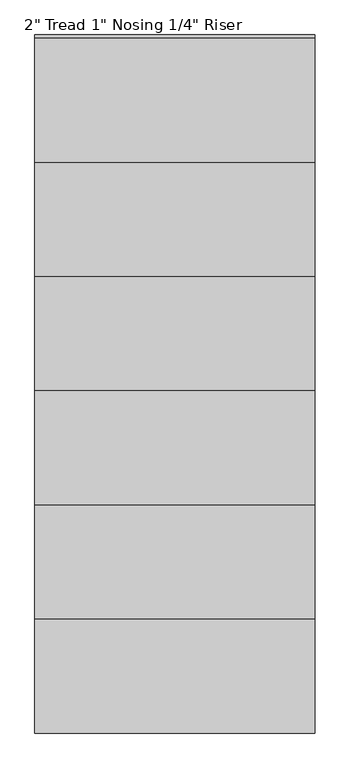
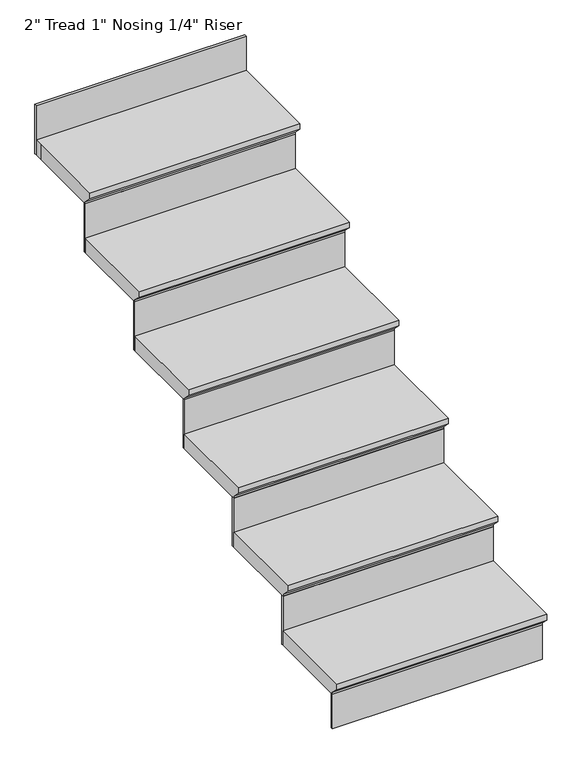
"""IFC4 building model written with IfcOpenShell, lengths in millimetres: stair flight geometry."""

from ifc_helpers import new_model, si_unit, origin, place, context, project, spatial, faceted_brep, source, transform, mapped, element, save


def stair_flight_b26bc1e7(model_context):
    return source(origin(), model_context, "Body", "Brep", [
        faceted_brep([(-9533.9292802, 7174.6516835, 150.2833333), (-9533.9292802, 7174.6516835, 169.3333333), (-10219.7292802, 7174.6516835, 169.3333333), (-10219.7292802, 7174.6516835, 150.2833333), (-9533.9292802, 7200.0516835, 124.8833333), (-10219.7292802, 7200.0516835, 124.8833333), (-9533.9292802, 7479.4516835, 169.3333333), (-10219.7292802, 7479.4516835, 169.3333333), (-10219.7292802, 7200.0516835, 118.5333333), (-10219.7292802, 7479.4516835, 118.5333333), (-9533.9292802, 7479.4516835, 118.5333333), (-9533.9292802, 7200.0516835, 118.5333333)], [[[0, 1, 2, 3]], [[4, 0, 3, 5]], [[2, 1, 6, 7]], [[8, 9, 10, 11]], [[2, 7, 9, 8, 5, 3]], [[8, 11, 4, 5]], [[6, 1, 0, 4, 11, 10]], [[7, 6, 10, 9]]]),
        faceted_brep([(-9533.9292802, 7200.0516835, 118.5333333), (-9533.9292802, 7200.0516835, 0.0), (-9533.9292802, 7206.4016835, 0.0), (-9533.9292802, 7206.4016835, 118.5333333), (-10219.7292802, 7200.0516835, 118.5333333), (-10219.7292802, 7206.4016835, 118.5333333), (-10219.7292802, 7206.4016835, 0.0), (-10219.7292802, 7200.0516835, 0.0)], [[[0, 1, 2, 3]], [[4, 5, 6, 7]], [[1, 0, 4, 7]], [[2, 1, 7, 6]], [[3, 2, 6, 5]], [[0, 3, 5, 4]]]),
        faceted_brep([(-9533.9292802, 7479.4516835, 287.8666667), (-9533.9292802, 7479.4516835, 118.5333333), (-9533.9292802, 7485.8016835, 118.5333333), (-9533.9292802, 7485.8016835, 287.8666667), (-10219.7292802, 7479.4516835, 287.8666667), (-10219.7292802, 7485.8016835, 287.8666667), (-10219.7292802, 7485.8016835, 118.5333333), (-10219.7292802, 7479.4516835, 118.5333333)], [[[0, 1, 2, 3]], [[4, 5, 6, 7]], [[1, 0, 4, 7]], [[2, 1, 7, 6]], [[3, 2, 6, 5]], [[0, 3, 5, 4]]]),
        faceted_brep([(-10219.7292802, 7454.0516835, 338.6666667), (-9533.9292802, 7454.0516835, 338.6666667), (-9533.9292802, 7758.8516835, 338.6666667), (-10219.7292802, 7758.8516835, 338.6666667), (-10219.7292802, 7479.4516835, 287.8666667), (-10219.7292802, 7758.8516835, 287.8666667), (-9533.9292802, 7758.8516835, 287.8666667), (-9533.9292802, 7479.4516835, 287.8666667), (-10219.7292802, 7479.4516835, 294.2166667), (-10219.7292802, 7454.0516835, 319.6166667), (-9533.9292802, 7479.4516835, 294.2166667), (-9533.9292802, 7454.0516835, 319.6166667)], [[[0, 1, 2, 3]], [[4, 5, 6, 7]], [[0, 3, 5, 4, 8, 9]], [[4, 7, 10, 8]], [[2, 1, 11, 10, 7, 6]], [[3, 2, 6, 5]], [[11, 1, 0, 9]], [[10, 11, 9, 8]]]),
        faceted_brep([(-9533.9292802, 7758.8516835, 457.2), (-9533.9292802, 7758.8516835, 287.8666667), (-9533.9292802, 7765.2016835, 287.8666667), (-9533.9292802, 7765.2016835, 457.2), (-10219.7292802, 7758.8516835, 457.2), (-10219.7292802, 7765.2016835, 457.2), (-10219.7292802, 7765.2016835, 287.8666667), (-10219.7292802, 7758.8516835, 287.8666667)], [[[0, 1, 2, 3]], [[4, 5, 6, 7]], [[1, 0, 4, 7]], [[2, 1, 7, 6]], [[3, 2, 6, 5]], [[0, 3, 5, 4]]]),
        faceted_brep([(-10219.7292802, 7733.4516835, 508.0), (-9533.9292802, 7733.4516835, 508.0), (-9533.9292802, 8038.2516835, 508.0), (-10219.7292802, 8038.2516835, 508.0), (-10219.7292802, 7758.8516835, 457.2), (-10219.7292802, 8038.2516835, 457.2), (-9533.9292802, 8038.2516835, 457.2), (-9533.9292802, 7758.8516835, 457.2), (-10219.7292802, 7758.8516835, 463.55), (-10219.7292802, 7733.4516835, 488.95), (-9533.9292802, 7758.8516835, 463.55), (-9533.9292802, 7733.4516835, 488.95)], [[[0, 1, 2, 3]], [[4, 5, 6, 7]], [[0, 3, 5, 4, 8, 9]], [[4, 7, 10, 8]], [[2, 1, 11, 10, 7, 6]], [[3, 2, 6, 5]], [[11, 1, 0, 9]], [[10, 11, 9, 8]]]),
        faceted_brep([(-9533.9292802, 8038.2516835, 626.5333333), (-9533.9292802, 8038.2516835, 457.2), (-9533.9292802, 8044.6016835, 457.2), (-9533.9292802, 8044.6016835, 626.5333333), (-10219.7292802, 8038.2516835, 626.5333333), (-10219.7292802, 8044.6016835, 626.5333333), (-10219.7292802, 8044.6016835, 457.2), (-10219.7292802, 8038.2516835, 457.2)], [[[0, 1, 2, 3]], [[4, 5, 6, 7]], [[1, 0, 4, 7]], [[2, 1, 7, 6]], [[3, 2, 6, 5]], [[0, 3, 5, 4]]]),
        faceted_brep([(-10219.7292802, 8012.8516835, 677.3333333), (-9533.9292802, 8012.8516835, 677.3333333), (-9533.9292802, 8317.6516835, 677.3333333), (-10219.7292802, 8317.6516835, 677.3333333), (-10219.7292802, 8038.2516835, 626.5333333), (-10219.7292802, 8317.6516835, 626.5333333), (-9533.9292802, 8317.6516835, 626.5333333), (-9533.9292802, 8038.2516835, 626.5333333), (-10219.7292802, 8038.2516835, 632.8833333), (-10219.7292802, 8012.8516835, 658.2833333), (-9533.9292802, 8038.2516835, 632.8833333), (-9533.9292802, 8012.8516835, 658.2833333)], [[[0, 1, 2, 3]], [[4, 5, 6, 7]], [[0, 3, 5, 4, 8, 9]], [[4, 7, 10, 8]], [[2, 1, 11, 10, 7, 6]], [[3, 2, 6, 5]], [[11, 1, 0, 9]], [[10, 11, 9, 8]]]),
        faceted_brep([(-9533.9292802, 8317.6516835, 795.8666667), (-9533.9292802, 8317.6516835, 626.5333333), (-9533.9292802, 8324.0016835, 626.5333333), (-9533.9292802, 8324.0016835, 795.8666667), (-10219.7292802, 8317.6516835, 795.8666667), (-10219.7292802, 8324.0016835, 795.8666667), (-10219.7292802, 8324.0016835, 626.5333333), (-10219.7292802, 8317.6516835, 626.5333333)], [[[0, 1, 2, 3]], [[4, 5, 6, 7]], [[1, 0, 4, 7]], [[2, 1, 7, 6]], [[3, 2, 6, 5]], [[0, 3, 5, 4]]]),
        faceted_brep([(-10219.7292802, 8292.2516835, 846.6666667), (-9533.9292802, 8292.2516835, 846.6666667), (-9533.9292802, 8597.0516835, 846.6666667), (-10219.7292802, 8597.0516835, 846.6666667), (-10219.7292802, 8317.6516835, 795.8666667), (-10219.7292802, 8597.0516835, 795.8666667), (-9533.9292802, 8597.0516835, 795.8666667), (-9533.9292802, 8317.6516835, 795.8666667), (-10219.7292802, 8317.6516835, 802.2166667), (-10219.7292802, 8292.2516835, 827.6166667), (-9533.9292802, 8317.6516835, 802.2166667), (-9533.9292802, 8292.2516835, 827.6166667)], [[[0, 1, 2, 3]], [[4, 5, 6, 7]], [[0, 3, 5, 4, 8, 9]], [[4, 7, 10, 8]], [[2, 1, 11, 10, 7, 6]], [[3, 2, 6, 5]], [[11, 1, 0, 9]], [[10, 11, 9, 8]]]),
        faceted_brep([(-9533.9292802, 8876.4516835, 1134.5333333), (-9533.9292802, 8876.4516835, 965.2), (-9533.9292802, 8882.8016835, 965.2), (-9533.9292802, 8882.8016835, 1134.5333333), (-10219.7292802, 8876.4516835, 1134.5333333), (-10219.7292802, 8882.8016835, 1134.5333333), (-10219.7292802, 8882.8016835, 965.2), (-10219.7292802, 8876.4516835, 965.2)], [[[0, 1, 2, 3]], [[4, 5, 6, 7]], [[1, 0, 4, 7]], [[2, 1, 7, 6]], [[3, 2, 6, 5]], [[0, 3, 5, 4]]]),
        faceted_brep([(-9533.9292802, 8597.0516835, 965.2), (-9533.9292802, 8597.0516835, 795.8666667), (-9533.9292802, 8603.4016835, 795.8666667), (-9533.9292802, 8603.4016835, 965.2), (-10219.7292802, 8597.0516835, 965.2), (-10219.7292802, 8603.4016835, 965.2), (-10219.7292802, 8603.4016835, 795.8666667), (-10219.7292802, 8597.0516835, 795.8666667)], [[[0, 1, 2, 3]], [[4, 5, 6, 7]], [[1, 0, 4, 7]], [[2, 1, 7, 6]], [[3, 2, 6, 5]], [[0, 3, 5, 4]]]),
        faceted_brep([(-10219.7292802, 8876.4516835, 1016.0), (-10219.7292802, 8851.0516835, 1016.0), (-10219.7292802, 8571.6516835, 1016.0), (-9533.9292802, 8571.6516835, 1016.0), (-9533.9292802, 8876.4516835, 1016.0), (-10219.7292802, 8851.0516835, 965.2), (-10219.7292802, 8876.4516835, 965.2), (-9533.9292802, 8876.4516835, 965.2), (-9533.9292802, 8597.0516835, 965.2), (-10219.7292802, 8597.0516835, 965.2), (-10219.7292802, 8597.0516835, 971.55), (-10219.7292802, 8571.6516835, 996.95), (-9533.9292802, 8597.0516835, 971.55), (-9533.9292802, 8571.6516835, 996.95)], [[[0, 1, 2, 3, 4]], [[5, 6, 7, 8, 9]], [[1, 0, 6, 5]], [[2, 1, 5, 9, 10, 11]], [[9, 8, 12, 10]], [[4, 3, 13, 12, 8, 7]], [[0, 4, 7, 6]], [[13, 3, 2, 11]], [[12, 13, 11, 10]]]),
    ])


if __name__ == "__main__":
    model = new_model("IFC4")
    model_context = context("Model", 3, world=origin())
    ifc_project = project(units=[si_unit("LENGTHUNIT", "METRE", prefix="MILLI")], contexts=[model_context])
    site = spatial("IfcSite", under=ifc_project)
    building = spatial("IfcBuilding", under=site)
    placement = place(None, origin())
    stair_flight_shape = stair_flight_b26bc1e7(model_context)
    element("IfcStairFlight", 1, ObjectType="2\" Tread 1\" Nosing 1/4\" Riser", at=placement, inside=building, context=model_context, shape_type="MappedRepresentation", body=[
        mapped(stair_flight_shape, transform((0.0, 0.0, 0.0), x_axis=(1.0, 0.0, 0.0), y_axis=(0.0, 1.0, 0.0), z_axis=(0.0, 0.0, 1.0))),
    ])
    save(model, "model.ifc")
